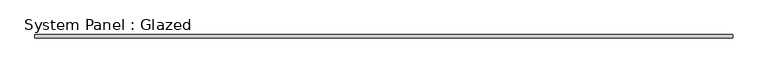
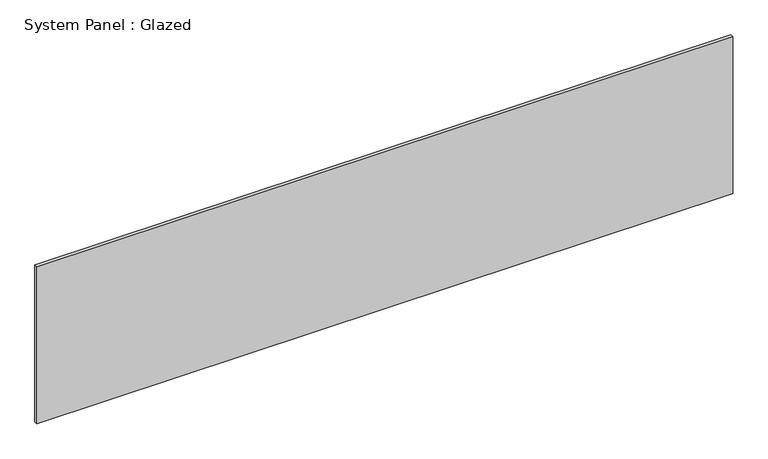
"""IFC4 building model written with IfcOpenShell, lengths in millimetres: plate geometry, System Panel : Glazed."""

from ifc_helpers import new_model, si_unit, origin, origin_with_axes, place, context, project, spatial, polyline, outline, extrude, source, transform, mapped, element, save


def system_panel_glazed_1e6177f2(model_context):
    return source(origin(), model_context, "Body", "SweptSolid", [
        extrude(outline(polyline([(2557.1124671, 19.05), (-2557.1124671, 19.05), (-2557.1124671, 44.45), (2557.1124671, 44.45), (2557.1124671, 19.05)])), origin_with_axes(), (0.0, 0.0, 1.0), 1219.2),
    ])


if __name__ == "__main__":
    model = new_model("IFC4")
    model_context = context("Model", 3, world=origin())
    ifc_project = project(units=[si_unit("LENGTHUNIT", "METRE", prefix="MILLI")], contexts=[model_context])
    site = spatial("IfcSite", under=ifc_project)
    building = spatial("IfcBuilding", under=site)
    placement = place(None, origin())
    system_panel_glazed_shape = system_panel_glazed_1e6177f2(model_context)
    element("IfcPlate", 1, ObjectType="System Panel : Glazed", at=placement, inside=building, context=model_context, shape_type="MappedRepresentation", body=[
        mapped(system_panel_glazed_shape, transform((0.0, 0.0, 0.0), x_axis=(1.0, 0.0, 0.0), y_axis=(0.0, 1.0, 0.0), z_axis=(0.0, 0.0, 1.0))),
    ])
    save(model, "model.ifc")

# Revit data of these elements
# Type "System Panel : Glazed"
#   Construction Type Id = "GSP4R"
#   Analytic Construction = "1/8 in Pilkington single glazing"
#   Visual Light Transmittance = 0.9
#   Solar Heat Gain Coefficient = 0.86
#   Heat Transfer Coefficient (U) = 1.18115 BTU/(h·ft²·°F)
# Element 1 (IfcPlate, "System Panel : Glazed")
#   Materials on its faces: "Glass"
# Materials
#   "Glass": class "Glass", colour RGB 0 128 192, transparency 0.75, Description = "Soda Lime Glass", Cost = 0
